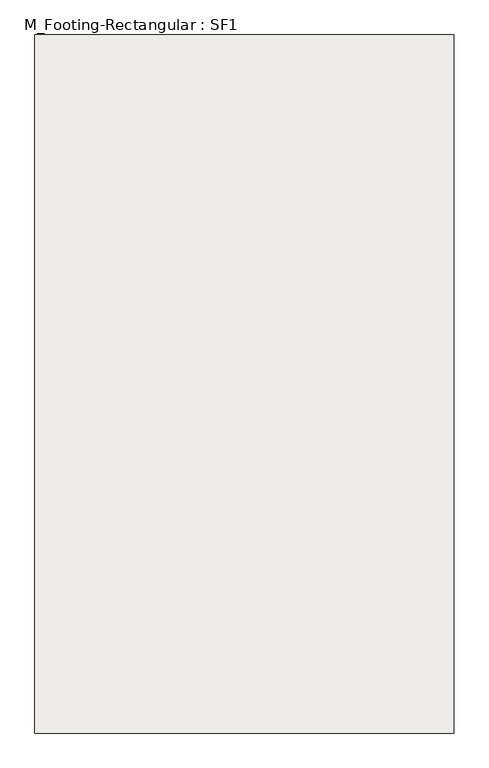
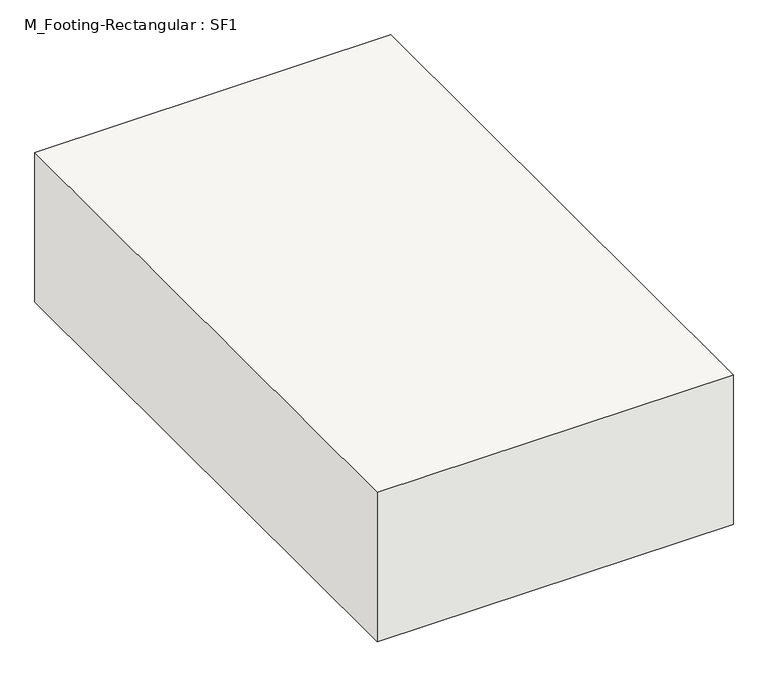
"""IFC4 building model written with IfcOpenShell, lengths in millimetres: slab geometry, M_Footing-Rectangular : SF1."""

from ifc_helpers import new_model, si_unit, frame, origin, place, context, project, spatial, polyline, outline, extrude, source, transform, mapped, element, save


def m_footing_rectangular_sf1_7ce3103a(model_context):
    return source(origin(), model_context, "Body", "SweptSolid", [
        extrude(outline(polyline([(685.8, 1143.0), (685.8, -1143.0), (-685.8, -1143.0), (-685.8, 1143.0), (685.8, 1143.0)])), frame((0.0, 0.0, -609.6), z_axis=(0.0, 0.0, 1.0), x_axis=(1.0, 0.0, 0.0)), (0.0, 0.0, 1.0), 609.6),
    ])


if __name__ == "__main__":
    model = new_model("IFC4")
    model_context = context("Model", 3, world=origin())
    ifc_project = project(units=[si_unit("LENGTHUNIT", "METRE", prefix="MILLI")], contexts=[model_context])
    site = spatial("IfcSite", under=ifc_project)
    building = spatial("IfcBuilding", under=site)
    placement = place(None, origin())
    m_footing_rectangular_sf1_shape = m_footing_rectangular_sf1_7ce3103a(model_context)
    element("IfcSlab", 1, ObjectType="M_Footing-Rectangular : SF1", at=placement, inside=building, context=model_context, shape_type="MappedRepresentation", body=[
        mapped(m_footing_rectangular_sf1_shape, transform((0.0, 0.0, 0.0), x_axis=(1.0, 0.0, 0.0), y_axis=(0.0, 1.0, 0.0), z_axis=(0.0, 0.0, 1.0))),
    ])
    save(model, "model.ifc")

# Revit data of these elements
# Type "M_Footing-Rectangular : SF1"
#   Width = 1371.6 mm
#   Length = 2286 mm
#   Foundation Thickness = 609.6 mm
#   Structural Material [instance default] = Concrete, Cast-in-Place gray
#   Assembly Code = ""
# Element 1 (IfcSlab, "M_Footing-Rectangular : SF1")
#   Materials on its faces: "Concrete, Cast-in-Place gray"
# Materials
#   "Concrete, Cast-in-Place gray": class "Concrete", colour RGB 192 192 192, transparency 0, Description = "Cast-in-place concrete", Cost = 0
